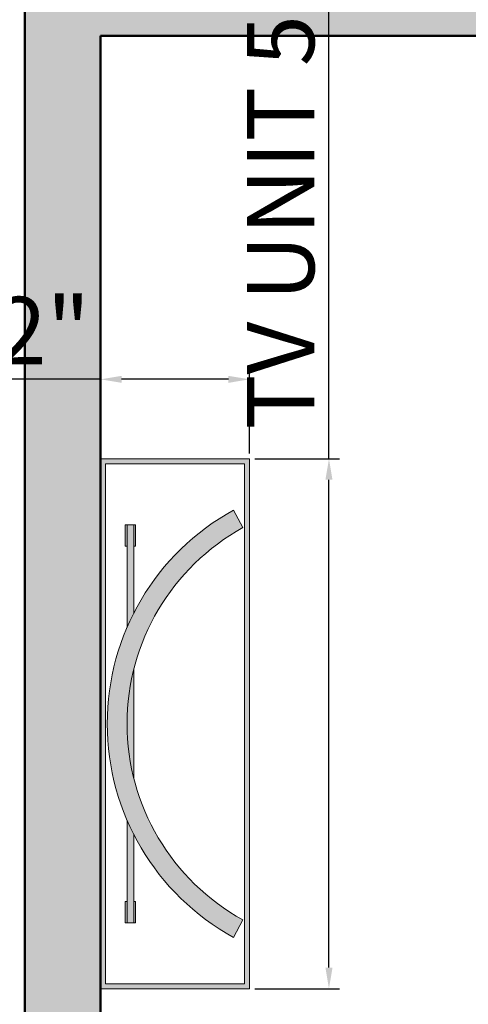
# Model space of a CAD drawing. Units: inches. Extents: x 3008 to 4088, y 1255 to 2137.
# Tile 7 of 30: x 3093 to 3146, y 1670 to 1787. Entities that reach past the tile are written whole.
import ezdxf

# ---------------------------------------------------------------- set-up
doc = ezdxf.new("R2010")
doc.units = ezdxf.units.IN
for name, color, linetype, lineweight in [('A-ANNO-DIMS', 2, 'Continuous', 18), ('A-FURN', 8, 'Continuous', 18), ('A-WALL', 7, 'Continuous', 50), ('A-WALL-PATT', 8, 'Continuous', 13), ('aparador', 36, 'Continuous', 9), ('moveis', 254, 'Continuous', 5)]:
    doc.layers.add(name, color=color, linetype=linetype, lineweight=lineweight)
doc.styles.get("Standard").update_dxf_attribs({"font": 'arial.ttf'})
doc.dimstyles.new('ISO-25', dxfattribs={"dimtxt": 8, "dimasz": 2.5, "dimexe": 1.25, "dimexo": 0.625, "dimtad": 1, "dimdec": 1, "dimlunit": 3, "dimtxsty": 'Standard', "dimcen": 2.5, "dimadec": 0, "dimazin": 0, "dimtfac": 1, "dimtdec": 1, "dimtmove": 0, "dimatfit": 3, "dimfxl": 1, "dimarcsym": 0})

# ---------------------------------------------------------------- blocks, each defined once
blk = doc.blocks.new('Aparador ORGANICA Formatto')
at = {"layer": 'aparador', "ltscale": 0.3}
h = blk.add_hatch(color=256, dxfattribs=at)
h.dxf.hatch_style = 1
h.set_gradient(color1=(118, 213, 123), color2=(52, 168, 57), one_color=1, tint=0.43, name='INVCURVED')
h.paths.add_polyline_path([(0.8, 0.45), (-0.8, 0.45), (-0.8, 0), (0.8, 0)])
h.paths.add_polyline_path([(0.785, 0.435), (0.785, 0.015), (-0.785, 0.015), (-0.785, 0.435)], flags=16)
h.paths.add_polyline_path([(0.2911, 0.3699), (0.5365, 0.3699), (0.5365, 0.3757), (0.6011, 0.3757), (0.6011, 0.3699), (0.6011, 0.3499), (0.6011, 0.3441), (0.5365, 0.3441), (0.5365, 0.3499), (0.3338, 0.3499, -0.150336), (0.6449, 0.0488), (0.5923, 0.0199, 0.208852), (0.1632, 0.3499), (-0.1632, 0.3499, 0.208852), (-0.5923, 0.0199), (-0.6449, 0.0488, -0.150336), (-0.3338, 0.3499), (-0.5365, 0.3499), (-0.5365, 0.3441), (-0.6011, 0.3441), (-0.6011, 0.3499), (-0.6011, 0.3699), (-0.6011, 0.3757), (-0.5365, 0.3757), (-0.5365, 0.3699), (-0.2911, 0.3699, -0.206106)], flags=0)
h = blk.add_hatch(color=256, dxfattribs=at)
h.dxf.hatch_style = 1
h.set_gradient(color1=(135, 92, 69), color2=(0, 0, 0), one_color=1, name='INVCURVED')
h.paths.add_polyline_path([(-0.6449, 0.0488), (-0.5923, 0.0199, -0.590888), (0.5923, 0.0199), (0.6449, 0.0488, 0.590888)])
h = blk.add_hatch(color=256, dxfattribs=at)
h.dxf.hatch_style = 1
h.set_gradient(color1=(178, 189, 189), one_color=1, tint=1, name='CYLINDER')
h.paths.add_polyline_path([(-0.5365, 0.3757), (-0.6011, 0.3757), (-0.6011, 0.3699), (-0.5365, 0.3699)])
h.paths.add_polyline_path([(-0.5365, 0.3499), (-0.6011, 0.3499), (-0.6011, 0.3441), (-0.5365, 0.3441)])
h = blk.add_hatch(color=256, dxfattribs=at)
h.dxf.hatch_style = 1
h.set_gradient(color1=(118, 213, 123), color2=(31, 101, 35), one_color=1, tint=0.26, name='INVCURVED')
h.paths.add_polyline_path([(-0.2911, 0.3699), (-0.6011, 0.3699), (-0.6011, 0.3499), (-0.3338, 0.3499, -0.015999)])
h = blk.add_hatch(color=256, dxfattribs=at)
h.dxf.hatch_style = 1
h.set_gradient(color1=(118, 213, 123), color2=(31, 101, 35), one_color=1, tint=0.26, name='INVCURVED')
h.paths.add_polyline_path([(-0.1632, 0.3499), (0.1632, 0.3499, 0.122516)])
h = blk.add_hatch(color=256, dxfattribs=at)
h.dxf.hatch_style = 1
h.set_gradient(color1=(118, 213, 123), color2=(31, 101, 35), one_color=1, tint=0.26, name='INVCURVED')
h.paths.add_polyline_path([(0.6011, 0.3699), (0.2911, 0.3699, -0.015999), (0.3338, 0.3499), (0.6011, 0.3499)])
h = blk.add_hatch(color=256, dxfattribs=at)
h.dxf.hatch_style = 1
h.set_gradient(color1=(178, 189, 189), one_color=1, tint=1, name='CYLINDER')
h.paths.add_polyline_path([(0.6011, 0.3757), (0.5365, 0.3757), (0.5365, 0.3699), (0.6011, 0.3699)])
h.paths.add_polyline_path([(0.6011, 0.3499), (0.5365, 0.3499), (0.5365, 0.3441), (0.6011, 0.3441)])
for p, q in [((-0.5923, 0.0199), (-0.6449, 0.0488)), ((0.5923, 0.0199), (0.6449, 0.0488))]:
    blk.add_line(p, q, dxfattribs=at)
for points in [[(-0.6011, 0.3699), (-0.6011, 0.3757), (-0.5365, 0.3757), (-0.5365, 0.3699)], [(0.6011, 0.3699), (0.6011, 0.3757), (0.5365, 0.3757), (0.5365, 0.3699)], [(-0.5365, 0.3499), (-0.5365, 0.3441), (-0.6011, 0.3441), (-0.6011, 0.3499)], [(0.5365, 0.3499), (0.5365, 0.3441), (0.6011, 0.3441), (0.6011, 0.3499)]]:
    blk.add_lwpolyline(points, dxfattribs=at)
for radius in [0.7362, 0.6762]:
    blk.add_arc((0, -0.3063), radius, 28.8434, 151.1566, dxfattribs=at)
at = {"layer": 'moveis', "ltscale": 0.3}
for p, q in [((-0.6011, 0.3699), (-0.6011, 0.3499)), ((-0.2911, 0.3699), (-0.6011, 0.3699)), ((0.2911, 0.3699), (0.6011, 0.3699)), ((0.6011, 0.3699), (0.6011, 0.3499)), ((-0.6011, 0.3499), (-0.3338, 0.3499)), ((-0.1632, 0.3499), (0.1632, 0.3499)), ((0.6011, 0.3499), (0.3338, 0.3499))]:
    blk.add_line(p, q, dxfattribs=at)
for points in [[(-0.8, 0), (0.8, 0), (0.8, 0.45), (-0.8, 0.45)], [(-0.785, 0.015), (0.785, 0.015), (0.785, 0.435), (-0.785, 0.435)]]:
    blk.add_lwpolyline(points, close=True, dxfattribs=at)
blk = doc.blocks.new('*D71')
at = {"layer": 'A-ANNO-DIMS', "color": 0, "lineweight": -2, "transparency": 16777216}
for p, q in [((3129.83, 1734.67), (3129.83, 1806.45)), ((3121.01, 1734.67), (3131.08, 1734.67)), ((3129.83, 1674.18), (3129.83, 1732.17)), ((3121.01, 1671.68), (3131.08, 1671.68))]:
    blk.add_line(p, q, dxfattribs=at)
at = {"layer": 'A-ANNO-DIMS', "color": 0, "transparency": 16777216}
for points in [[(3129.41, 1732.17), (3130.25, 1732.17), (3129.83, 1734.67)], [(3129.41, 1674.18), (3130.25, 1674.18), (3129.83, 1671.68)]]:
    blk.add_solid(points, dxfattribs=at)
at = {"layer": 'Defpoints', "color": 0, "transparency": 16777216}
for p in [(3120.38, 1734.67), (3129.83, 1734.67), (3120.38, 1671.68)]:
    blk.add_point(p, dxfattribs=at)
at = {"layer": 'A-ANNO-DIMS', "color": 0, "transparency": 16777216, "insert": (3125.12, 1771.81), "char_height": 8, "attachment_point": 5, "rotation": 90}
blk.add_mtext('TV UNIT 5\'-3"', dxfattribs=at)
blk = doc.blocks.new('*D72')
at = {"layer": 'A-ANNO-DIMS', "color": 0, "lineweight": -2, "transparency": 16777216}
for p, q in [((3102.67, 1735.29), (3102.67, 1745.37)), ((3120.38, 1735.29), (3120.38, 1745.37)), ((3102.67, 1744.12), (3059.76, 1744.12)), ((3117.88, 1744.12), (3105.17, 1744.12))]:
    blk.add_line(p, q, dxfattribs=at)
at = {"layer": 'A-ANNO-DIMS', "color": 0, "transparency": 16777216}
for points in [[(3105.17, 1744.53), (3105.17, 1743.7), (3102.67, 1744.12)], [(3117.88, 1744.53), (3117.88, 1743.7), (3120.38, 1744.12)]]:
    blk.add_solid(points, dxfattribs=at)
at = {"layer": 'Defpoints', "color": 0, "transparency": 16777216}
for p in [(3102.67, 1744.12), (3102.67, 1734.67), (3120.38, 1734.67)]:
    blk.add_point(p, dxfattribs=at)
at = {"layer": 'A-ANNO-DIMS', "color": 0, "transparency": 16777216, "insert": (3079.96, 1748.88), "char_height": 8, "attachment_point": 5}
blk.add_mtext('1\'-5 1/2"', dxfattribs=at)

msp = doc.modelspace()

# ---------------------------------------------------------------- hatches: boundary and pattern name
at = {"layer": 'A-WALL-PATT'}
h = msp.add_hatch(color=256, dxfattribs=at)
h.dxf.hatch_style = 1
h.paths.add_polyline_path([(3102.67, 1625.97), (3093.67, 1625.97), (3093.67, 1540.97), (3102.67, 1540.97)])
h.paths.add_polyline_path([(3102.67, 1784.97), (3252.67, 1784.97), (3252.67, 1790.97), (3102.67, 1790.97), (3102.67, 1892.97), (3093.67, 1892.97), (3093.67, 1667.97), (3102.67, 1667.97)])
h.paths.add_polyline_path([(3192.67, 1943.97), (3093.67, 1943.97), (3093.67, 1934.97), (3102.67, 1934.97), (3192.67, 1934.97)])
h.paths.add_polyline_path([(3264.67, 1943.97), (3234.67, 1943.97), (3234.67, 1934.97), (3246.67, 1934.97), (3246.67, 1868.97), (3252.67, 1868.97), (3252.67, 1934.97), (3264.67, 1934.97)])
h.paths.add_polyline_path([(3330.67, 1943.97), (3288.67, 1943.97), (3288.67, 1934.97), (3300.67, 1934.97), (3300.67, 1838.97), (3246.67, 1838.97), (3246.67, 1826.97), (3252.67, 1826.97), (3252.67, 1832.97), (3306.67, 1832.97), (3306.67, 1934.97), (3330.67, 1934.97)])
h.paths.add_polyline_path([(3390.67, 1943.97), (3360.67, 1943.97), (3360.67, 1934.97), (3390.67, 1934.97)])
h.paths.add_polyline_path([(3465.67, 1943.97), (3432.67, 1943.97), (3432.67, 1934.97), (3456.67, 1934.97), (3456.67, 1883.97), (3465.67, 1883.97)])
h.paths.add_polyline_path([(3465.67, 1841.97), (3456.67, 1841.97), (3456.67, 1790.97), (3370.67, 1790.97), (3370.67, 1784.97), (3456.67, 1784.97), (3456.67, 1759.47), (3465.67, 1759.47)])
h.paths.add_polyline_path([(3465.67, 1693.47), (3456.67, 1693.47), (3456.67, 1667.97), (3330.67, 1667.97), (3330.67, 1643.97), (3336.67, 1643.97), (3336.67, 1661.97), (3456.67, 1661.97), (3456.67, 1649.97), (3465.67, 1649.97)])
h.paths.add_polyline_path([(3465.67, 1625.97), (3456.67, 1625.97), (3456.67, 1613.97), (3324.67, 1613.97), (3324.67, 1604.97), (3456.67, 1604.97), (3456.67, 1571.97), (3465.67, 1571.97)])
h.paths.add_polyline_path([(3465.67, 1505.97), (3456.67, 1505.97), (3456.67, 1472.97), (3438.67, 1472.97), (3438.67, 1463.97), (3465.67, 1463.97)])
h.paths.add_polyline_path([(3396.67, 1472.97), (3354.67, 1472.97), (3354.67, 1463.97), (3396.67, 1463.97)])
h.paths.add_polyline_path([(3312.67, 1472.97), (3288.67, 1472.97), (3288.67, 1550.97), (3282.67, 1550.97), (3282.67, 1472.97), (3270.67, 1472.97), (3270.67, 1463.97), (3312.67, 1463.97)])
h.paths.add_polyline_path([(3246.67, 1472.97), (3234.67, 1472.97), (3234.67, 1544.97), (3252.67, 1544.97), (3252.67, 1550.97), (3234.67, 1550.97), (3234.67, 1604.97), (3282.67, 1604.97), (3282.67, 1580.97), (3288.67, 1580.97), (3288.67, 1613.97), (3150.67, 1613.97), (3150.67, 1604.97), (3225.67, 1604.97), (3225.67, 1463.97), (3246.67, 1463.97)])

# ---------------------------------------------------------------- linework, layer by layer
at = {"layer": 'A-WALL'}
for p, q in [((3093.67, 1540.97), (3093.67, 1943.97)), ((3102.67, 1540.97), (3102.67, 1784.97)), ((3102.67, 1784.97), (3252.67, 1784.97))]:
    msp.add_line(p, q, dxfattribs=at)

# ---------------------------------------------------------------- block references
at = {"layer": 'A-FURN', "xscale": 39.3701, "yscale": 39.3701, "zscale": 39.3701, "rotation": 90}
msp.add_blockref('Aparador ORGANICA Formatto', (3120.38, 1703.17), dxfattribs=at)

# ---------------------------------------------------------------- dimensions: what is measured, and where the dimension line sits
at = {"layer": 'A-ANNO-DIMS'}
dim = msp.add_linear_dim(base=(3129.83, 1734.67), p1=(3120.38, 1671.68), p2=(3120.38, 1734.67), angle=90, text='TV UNIT <>', dimstyle='ISO-25', override={"dimdec": 1, "dimrnd": 0, "dimzin": 1, "dimlunit": 4, "dimfrac": 2}, dxfattribs=at)
dim.commit()
dim.dimension.update_dxf_attribs({"geometry": '*D71', "text_midpoint": (3125.12, 1771.81)})
dim = msp.add_linear_dim(base=(3102.67, 1744.12), p1=(3120.38, 1734.67), p2=(3102.67, 1734.67), angle=180, dimstyle='ISO-25', override={"dimdec": 1, "dimrnd": 0, "dimzin": 1, "dimlunit": 4, "dimfrac": 2}, dxfattribs=at)
dim.commit()
dim.dimension.update_dxf_attribs({"geometry": '*D72', "text_midpoint": (3079.96, 1748.88)})

doc.saveas('drawing.dxf')
